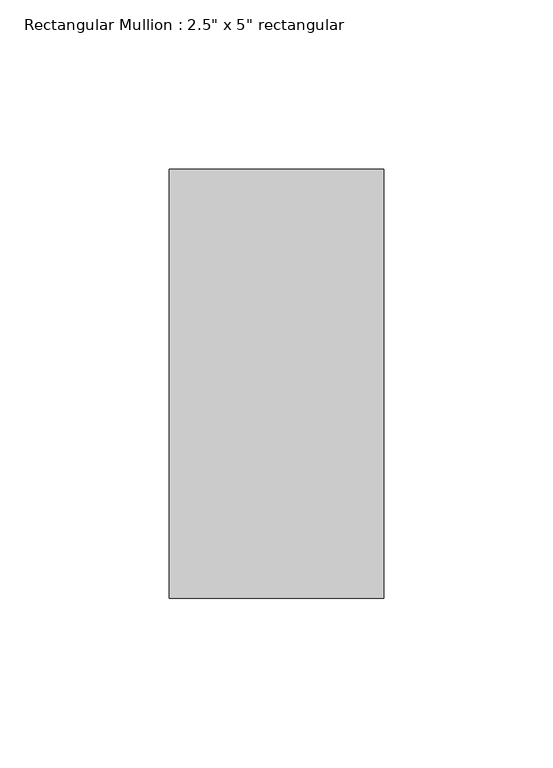
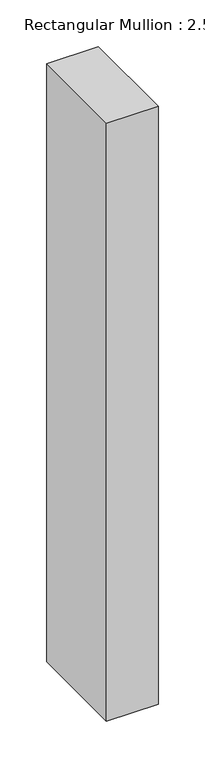
"""IFC4 building model written with IfcOpenShell, lengths in millimetres: member geometry."""

from ifc_helpers import new_model, si_unit, frame, origin, place, context, project, spatial, polyline, outline, extrude, source, transform, mapped, element, save


def member_32677b83(model_context):
    return source(origin(), model_context, "Body", "SweptSolid", [
        extrude(outline(polyline([(31.75, 63.5), (31.75, -63.5), (-31.75, -63.5), (-31.75, 63.5), (31.75, 63.5)])), frame((0.0, 0.0, -778.426051), z_axis=(0.0, 0.0, 1.0), x_axis=(1.0, 0.0, 0.0)), (0.0, 0.0, 1.0), 778.426051),
    ])


if __name__ == "__main__":
    model = new_model("IFC4")
    model_context = context("Model", 3, world=origin())
    ifc_project = project(units=[si_unit("LENGTHUNIT", "METRE", prefix="MILLI")], contexts=[model_context])
    site = spatial("IfcSite", under=ifc_project)
    building = spatial("IfcBuilding", under=site)
    placement = place(None, origin())
    member_shape = member_32677b83(model_context)
    element("IfcMember", 1, ObjectType="Rectangular Mullion : 2.5\" x 5\" rectangular", at=placement, inside=building, context=model_context, shape_type="MappedRepresentation", body=[
        mapped(member_shape, transform((0.0, 0.0, 0.0), x_axis=(1.0, 0.0, 0.0), y_axis=(0.0, 1.0, 0.0), z_axis=(0.0, 0.0, 1.0))),
    ])
    save(model, "model.ifc")

# Revit data of these elements
# Type "Rectangular Mullion : 2.5\" x 5\" rectangular"
#   built-in parameter 1007304 = 0.416667 (stored number, unit not read)
#   built-in parameter 1007301 = 0.104167 (stored number, unit not read)
#   built-in parameter 1007300 = 0.104167 (stored number, unit not read)
# Element 1 (IfcMember, "Rectangular Mullion : 2.5\" x 5\" rectangular")
#   Materials on its faces: "Aluminum"
# Materials
#   "Aluminum": class "Metal", colour RGB 247 247 247, transparency 0, Description = "Aluminum 6061", Cost = 0
